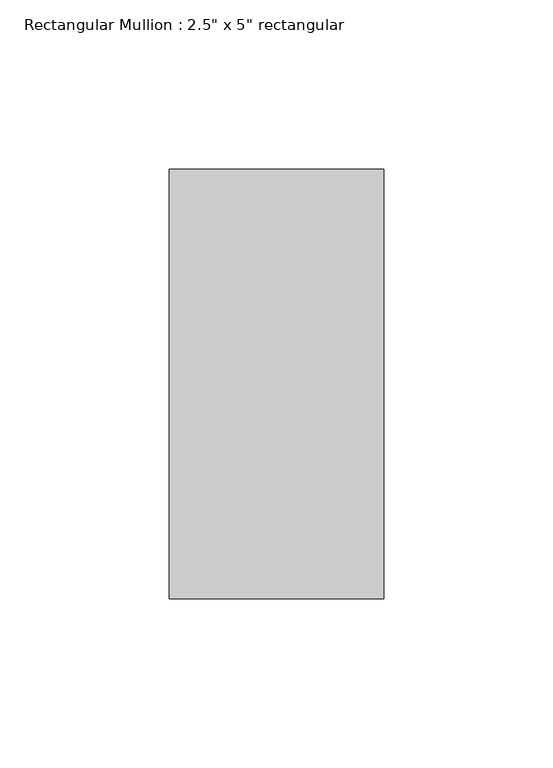
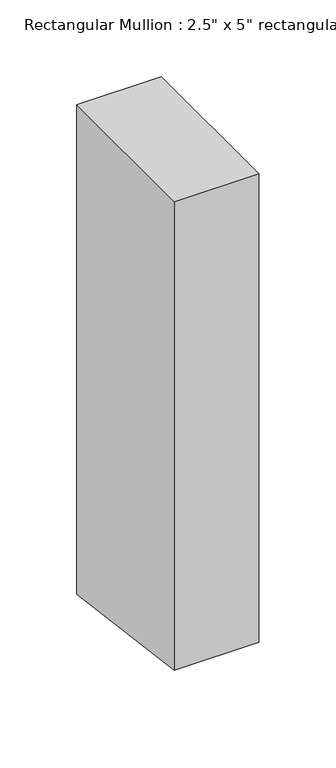
"""IFC4 building model written with IfcOpenShell, lengths in millimetres: member geometry."""

from ifc_helpers import new_model, si_unit, frame, origin, place, context, project, spatial, polyline, outline, extrude, source, transform, mapped, element, save


def member_f1972444(model_context):
    return source(origin(), model_context, "Body", "SweptSolid", [
        extrude(outline(polyline([(-63.5, 0.0), (63.5, 0.0), (63.5, -388.8541629), (-63.5, -372.3871146), (-63.5, 0.0)])), frame((-63.5, 0.0, 0.0), z_axis=(1.0, 0.0, 0.0), x_axis=(0.0, 1.0, 0.0)), (0.0, 0.0, 1.0), 63.5),
    ])


if __name__ == "__main__":
    model = new_model("IFC4")
    model_context = context("Model", 3, world=origin())
    ifc_project = project(units=[si_unit("LENGTHUNIT", "METRE", prefix="MILLI")], contexts=[model_context])
    site = spatial("IfcSite", under=ifc_project)
    building = spatial("IfcBuilding", under=site)
    placement = place(None, origin())
    member_shape = member_f1972444(model_context)
    element("IfcMember", 1, ObjectType="Rectangular Mullion : 2.5\" x 5\" rectangular", at=placement, inside=building, context=model_context, shape_type="MappedRepresentation", body=[
        mapped(member_shape, transform((0.0, 0.0, 0.0), x_axis=(1.0, 0.0, 0.0), y_axis=(0.0, 1.0, 0.0), z_axis=(0.0, 0.0, 1.0))),
    ])
    save(model, "model.ifc")

# Revit data of these elements
# Type "Rectangular Mullion : 2.5\" x 5\" rectangular"
#   built-in parameter 1007304 = 0.416667 (stored number, unit not read)
#   built-in parameter 1007301 = 0.104167 (stored number, unit not read)
#   built-in parameter 1007300 = 0.104167 (stored number, unit not read)
# Element 1 (IfcMember, "Rectangular Mullion : 2.5\" x 5\" rectangular")
#   Materials on its faces: "Iron, Ductile"
# Materials
#   "Iron, Ductile": class "Metal", colour RGB 0 0 0, transparency 0, Description = "Ductile cast iron", Cost = 0
